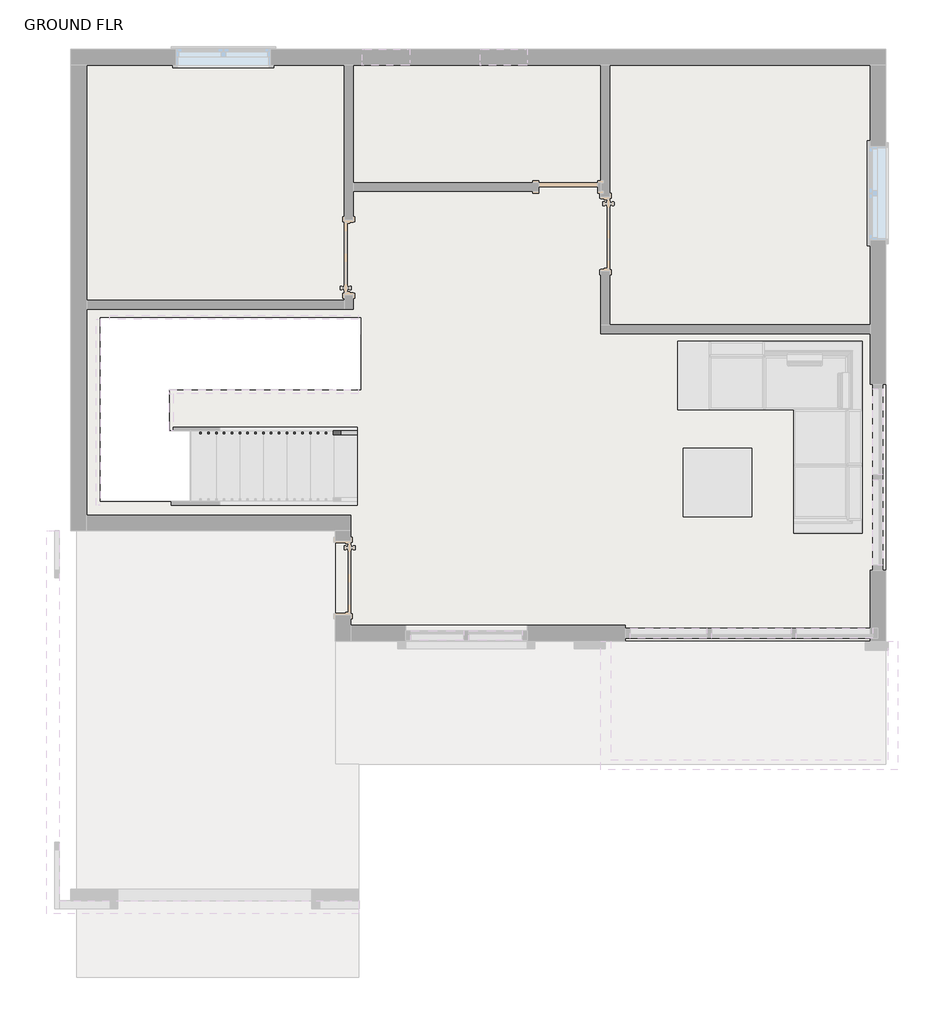
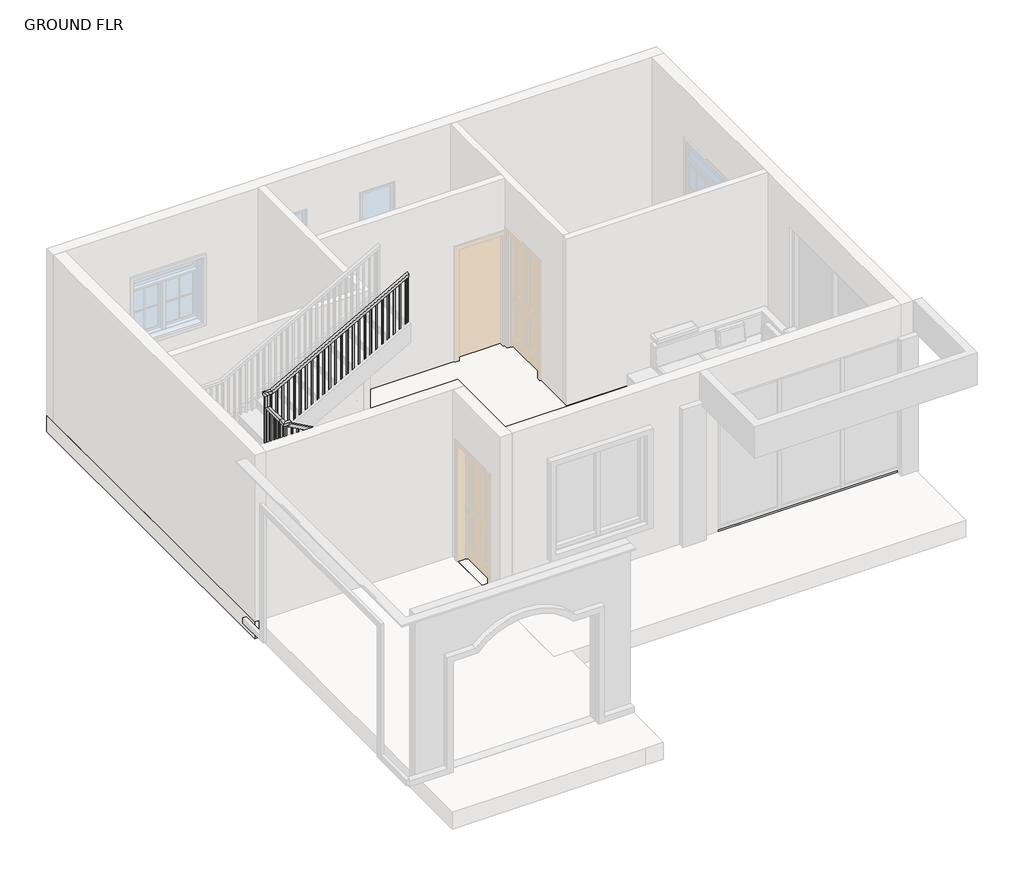
# One storey, part 2 of 3: 3 slabs, 1 beam, 1 railing.
"""IFC4 building model written with IfcOpenShell, lengths in millimetres."""

from ifc_helpers import new_model, si_unit, frame, origin, origin_with_axes, place, context, project, spatial, polyline, outline, extrude, faceted_brep, element, save

model = new_model("IFC4")

# Units and contexts
model_context = context("Model", 3, world=origin())
ifc_project = project(units=[si_unit("LENGTHUNIT", "METRE", prefix="MILLI")], contexts=[model_context])

# Site, building, storey
site = spatial("IfcSite", under=ifc_project)
building = spatial("IfcBuilding", under=site)
storey = spatial("IfcBuildingStorey", under=building, Name="GROUND FLR", Elevation=304.8)

# Beam
placement = place(None, origin())
element("IfcBeam", 1, ObjectType="Concrete-Rectangular Beam : 12 x 24", at=placement, inside=storey, context=model_context, shape_type="Brep", body=[
    faceted_brep([(-11339.0293601, -13183.002305, 304.8), (-11339.0293601, -13487.802305, 304.8), (-8226.1270642, -13487.802305, 304.8), (-8226.1270642, -13183.002305, 304.8), (-11339.0293601, -13183.002305, -304.8), (-11339.0293601, -13183.002305, 0.0), (-8226.1270642, -13183.002305, 0.0), (-8226.1270642, -13183.002305, -304.8), (-11339.0293601, -13487.802305, -304.8), (-8226.1270642, -13487.802305, -304.8), (-11339.0293601, -13487.802305, 0.0), (-8226.1270642, -13487.802305, 0.0)], [[[0, 1, 2, 3]], [[4, 5, 0, 3, 6, 7]], [[8, 4, 7, 9]], [[1, 10, 8, 9, 11, 2]], [[2, 11, 9, 7, 6, 3]], [[1, 0, 5, 4, 8, 10]]]),
])

# Railing
element("IfcRailing", 2, ObjectType="Handrail - Rectangular", at=placement, inside=storey, context=model_context, shape_type="SolidModel", body=[
    faceted_brep([(-7930.9736584, -7598.0396616, 1388.5333333), (-7930.9736584, -7598.0396616, 1330.420221), (-7930.9736584, -7547.2396616, 1330.420221), (-7930.9736584, -7547.2396616, 1388.5333333), (-10293.1736584, -7598.0396616, 2700.8666667), (-10343.9736584, -7598.0396616, 2670.9757765), (-10343.9736584, -7547.2396616, 2670.9757765), (-10293.1736584, -7547.2396616, 2700.8666667), (-10293.1736584, -7598.0396616, 2743.2), (-10343.9736584, -7598.0396616, 2692.4), (-10343.9736584, -7547.2396616, 2692.4), (-10293.1736584, -7547.2396616, 2743.2), (-10420.1736584, -7598.0396616, 2743.2), (-10420.1736584, -7598.0396616, 2692.4), (-10369.3736584, -7547.2396616, 2692.4), (-10369.3736584, -7547.2396616, 2743.2), (-10420.1736584, -7471.0396616, 2743.2), (-10420.1736584, -7471.0396616, 2692.4), (-10369.3736584, -7471.0396616, 2692.4), (-10369.3736584, -7471.0396616, 2743.2), (-10420.1736584, -7090.0396616, 2743.2), (-10420.1736584, -7039.2396616, 2692.4), (-10369.3736584, -7039.2396616, 2692.4), (-10369.3736584, -7090.0396616, 2743.2), (-10420.1736584, -7090.0396616, 2949.5074477), (-10420.1736584, -7039.2396616, 2898.7074477), (-10369.3736584, -7039.2396616, 2898.7074477), (-10369.3736584, -7090.0396616, 2949.5074477), (-10420.1736584, -6963.0396616, 2949.5074477), (-10420.1736584, -6963.0396616, 2898.7074477), (-10369.3736584, -7013.8396616, 2898.7074477), (-10369.3736584, -7013.8396616, 2949.5074477), (-10293.1736584, -6963.0396616, 2949.5074477), (-10280.0100562, -6963.0396616, 2898.7074477), (-10280.0100562, -7013.8396616, 2898.7074477), (-10293.1736584, -7013.8396616, 2949.5074477), (-7921.3270642, -6963.0396616, 4267.2), (-7921.3270642, -7013.8396616, 4267.2), (-7921.3270642, -7013.8396616, 4209.0868876), (-7921.3270642, -6963.0396616, 4209.0868876)], [[[0, 1, 2, 3]], [[1, 0, 4, 5]], [[2, 1, 5, 6]], [[3, 2, 6, 7]], [[0, 3, 7, 4]], [[5, 4, 8, 9]], [[6, 5, 9, 10]], [[7, 6, 10, 11]], [[4, 7, 11, 8]], [[9, 8, 12, 13]], [[10, 9, 13, 14]], [[11, 10, 14, 15]], [[8, 11, 15, 12]], [[13, 12, 16, 17]], [[14, 13, 17, 18]], [[15, 14, 18, 19]], [[12, 15, 19, 16]], [[17, 16, 20, 21]], [[18, 17, 21, 22]], [[19, 18, 22, 23]], [[16, 19, 23, 20]], [[21, 20, 24, 25]], [[22, 21, 25, 26]], [[23, 22, 26, 27]], [[20, 23, 27, 24]], [[25, 24, 28, 29]], [[26, 25, 29, 30]], [[27, 26, 30, 31]], [[24, 27, 31, 28]], [[29, 28, 32, 33]], [[30, 29, 33, 34]], [[31, 30, 34, 35]], [[28, 31, 35, 32]], [[36, 37, 38, 39]], [[33, 32, 36, 39]], [[34, 33, 39, 38]], [[35, 34, 38, 37]], [[32, 35, 37, 36]]]),
    extrude(outline(polyline([(4194.9082242, -7946.8486584), (4184.3248909, -7965.8986584), (3183.4666667, -7965.8986584), (3183.4666667, -7946.8486584), (4194.9082242, -7946.8486584)])), frame((0.0, -6997.9646616, 0.0), z_axis=(0.0, 1.0, 0.0), x_axis=(0.0, 0.0, 1.0)), (0.0, 0.0, 1.0), 19.05),
    extrude(outline(polyline([(4138.4637797, -8048.4486584), (4127.8804464, -8067.4986584), (3183.4666667, -8067.4986584), (3183.4666667, -8048.4486584), (4138.4637797, -8048.4486584)])), frame((0.0, -6997.9646616, 0.0), z_axis=(0.0, 1.0, 0.0), x_axis=(0.0, 0.0, 1.0)), (0.0, 0.0, 1.0), 19.05),
    extrude(outline(polyline([(4082.0193353, -8150.0486584), (4071.436002, -8169.0986584), (3183.4666667, -8169.0986584), (3183.4666667, -8150.0486584), (4082.0193353, -8150.0486584)])), frame((0.0, -6997.9646616, 0.0), z_axis=(0.0, 1.0, 0.0), x_axis=(0.0, 0.0, 1.0)), (0.0, 0.0, 1.0), 19.05),
    extrude(outline(polyline([(4025.5748909, -8251.6486584), (4014.9915575, -8270.6986584), (3014.1333333, -8270.6986584), (3014.1333333, -8251.6486584), (4025.5748909, -8251.6486584)])), frame((0.0, -6997.9646616, 0.0), z_axis=(0.0, 1.0, 0.0), x_axis=(0.0, 0.0, 1.0)), (0.0, 0.0, 1.0), 19.05),
    extrude(outline(polyline([(3969.1304464, -8353.2486584), (3958.5471131, -8372.2986584), (3014.1333333, -8372.2986584), (3014.1333333, -8353.2486584), (3969.1304464, -8353.2486584)])), frame((0.0, -6997.9646616, 0.0), z_axis=(0.0, 1.0, 0.0), x_axis=(0.0, 0.0, 1.0)), (0.0, 0.0, 1.0), 19.05),
    extrude(outline(polyline([(3912.686002, -8454.8486584), (3902.1026686, -8473.8986584), (3014.1333333, -8473.8986584), (3014.1333333, -8454.8486584), (3912.686002, -8454.8486584)])), frame((0.0, -6997.9646616, 0.0), z_axis=(0.0, 1.0, 0.0), x_axis=(0.0, 0.0, 1.0)), (0.0, 0.0, 1.0), 19.05),
    extrude(outline(polyline([(3856.2415575, -8556.4486584), (3845.6582242, -8575.4986584), (2844.8, -8575.4986584), (2844.8, -8556.4486584), (3856.2415575, -8556.4486584)])), frame((0.0, -6997.9646616, 0.0), z_axis=(0.0, 1.0, 0.0), x_axis=(0.0, 0.0, 1.0)), (0.0, 0.0, 1.0), 19.05),
    extrude(outline(polyline([(3799.7971131, -8658.0486584), (3789.2137797, -8677.0986584), (2844.8, -8677.0986584), (2844.8, -8658.0486584), (3799.7971131, -8658.0486584)])), frame((0.0, -6997.9646616, 0.0), z_axis=(0.0, 1.0, 0.0), x_axis=(0.0, 0.0, 1.0)), (0.0, 0.0, 1.0), 19.05),
    extrude(outline(polyline([(3743.3526686, -8759.6486584), (3732.7693353, -8778.6986584), (2844.8, -8778.6986584), (2844.8, -8759.6486584), (3743.3526686, -8759.6486584)])), frame((0.0, -6997.9646616, 0.0), z_axis=(0.0, 1.0, 0.0), x_axis=(0.0, 0.0, 1.0)), (0.0, 0.0, 1.0), 19.05),
    extrude(outline(polyline([(3686.9082242, -8861.2486584), (3676.3248909, -8880.2986584), (2675.4666667, -8880.2986584), (2675.4666667, -8861.2486584), (3686.9082242, -8861.2486584)])), frame((0.0, -6997.9646616, 0.0), z_axis=(0.0, 1.0, 0.0), x_axis=(0.0, 0.0, 1.0)), (0.0, 0.0, 1.0), 19.05),
    extrude(outline(polyline([(3630.4637797, -8962.8486584), (3619.8804464, -8981.8986584), (2675.4666667, -8981.8986584), (2675.4666667, -8962.8486584), (3630.4637797, -8962.8486584)])), frame((0.0, -6997.9646616, 0.0), z_axis=(0.0, 1.0, 0.0), x_axis=(0.0, 0.0, 1.0)), (0.0, 0.0, 1.0), 19.05),
    extrude(outline(polyline([(3574.0193353, -9064.4486584), (3563.436002, -9083.4986584), (2675.4666667, -9083.4986584), (2675.4666667, -9064.4486584), (3574.0193353, -9064.4486584)])), frame((0.0, -6997.9646616, 0.0), z_axis=(0.0, 1.0, 0.0), x_axis=(0.0, 0.0, 1.0)), (0.0, 0.0, 1.0), 19.05),
    extrude(outline(polyline([(3517.5748909, -9166.0486584), (3506.9915575, -9185.0986584), (2506.1333333, -9185.0986584), (2506.1333333, -9166.0486584), (3517.5748909, -9166.0486584)])), frame((0.0, -6997.9646616, 0.0), z_axis=(0.0, 1.0, 0.0), x_axis=(0.0, 0.0, 1.0)), (0.0, 0.0, 1.0), 19.05),
    extrude(outline(polyline([(3461.1304464, -9267.6486584), (3450.5471131, -9286.6986584), (2506.1333333, -9286.6986584), (2506.1333333, -9267.6486584), (3461.1304464, -9267.6486584)])), frame((0.0, -6997.9646616, 0.0), z_axis=(0.0, 1.0, 0.0), x_axis=(0.0, 0.0, 1.0)), (0.0, 0.0, 1.0), 19.05),
    extrude(outline(polyline([(3404.686002, -9369.2486584), (3394.1026686, -9388.2986584), (2506.1333333, -9388.2986584), (2506.1333333, -9369.2486584), (3404.686002, -9369.2486584)])), frame((0.0, -6997.9646616, 0.0), z_axis=(0.0, 1.0, 0.0), x_axis=(0.0, 0.0, 1.0)), (0.0, 0.0, 1.0), 19.05),
    extrude(outline(polyline([(3348.2415575, -9470.8486584), (3337.6582242, -9489.8986584), (2336.8, -9489.8986584), (2336.8, -9470.8486584), (3348.2415575, -9470.8486584)])), frame((0.0, -6997.9646616, 0.0), z_axis=(0.0, 1.0, 0.0), x_axis=(0.0, 0.0, 1.0)), (0.0, 0.0, 1.0), 19.05),
    extrude(outline(polyline([(3291.7971131, -9572.4486584), (3281.2137797, -9591.4986584), (2336.8, -9591.4986584), (2336.8, -9572.4486584), (3291.7971131, -9572.4486584)])), frame((0.0, -6997.9646616, 0.0), z_axis=(0.0, 1.0, 0.0), x_axis=(0.0, 0.0, 1.0)), (0.0, 0.0, 1.0), 19.05),
    extrude(outline(polyline([(3235.3526686, -9674.0486584), (3224.7693353, -9693.0986584), (2336.8, -9693.0986584), (2336.8, -9674.0486584), (3235.3526686, -9674.0486584)])), frame((0.0, -6997.9646616, 0.0), z_axis=(0.0, 1.0, 0.0), x_axis=(0.0, 0.0, 1.0)), (0.0, 0.0, 1.0), 19.05),
    extrude(outline(polyline([(3178.9082242, -9775.6486584), (3168.3248909, -9794.6986584), (2167.4666667, -9794.6986584), (2167.4666667, -9775.6486584), (3178.9082242, -9775.6486584)])), frame((0.0, -6997.9646616, 0.0), z_axis=(0.0, 1.0, 0.0), x_axis=(0.0, 0.0, 1.0)), (0.0, 0.0, 1.0), 19.05),
    extrude(outline(polyline([(3122.4637797, -9877.2486584), (3111.8804464, -9896.2986584), (2167.4666667, -9896.2986584), (2167.4666667, -9877.2486584), (3122.4637797, -9877.2486584)])), frame((0.0, -6997.9646616, 0.0), z_axis=(0.0, 1.0, 0.0), x_axis=(0.0, 0.0, 1.0)), (0.0, 0.0, 1.0), 19.05),
    extrude(outline(polyline([(3066.0193353, -9978.8486584), (3055.436002, -9997.8986584), (2167.4666667, -9997.8986584), (2167.4666667, -9978.8486584), (3066.0193353, -9978.8486584)])), frame((0.0, -6997.9646616, 0.0), z_axis=(0.0, 1.0, 0.0), x_axis=(0.0, 0.0, 1.0)), (0.0, 0.0, 1.0), 19.05),
    extrude(outline(polyline([(3009.5748909, -10080.4486584), (2998.9915575, -10099.4986584), (1998.1333333, -10099.4986584), (1998.1333333, -10080.4486584), (3009.5748909, -10080.4486584)])), frame((0.0, -6997.9646616, 0.0), z_axis=(0.0, 1.0, 0.0), x_axis=(0.0, 0.0, 1.0)), (0.0, 0.0, 1.0), 19.05),
    extrude(outline(polyline([(2953.1304464, -10182.0486584), (2942.5471131, -10201.0986584), (1998.1333333, -10201.0986584), (1998.1333333, -10182.0486584), (2953.1304464, -10182.0486584)])), frame((0.0, -6997.9646616, 0.0), z_axis=(0.0, 1.0, 0.0), x_axis=(0.0, 0.0, 1.0)), (0.0, 0.0, 1.0), 19.05),
    extrude(outline(polyline([(2896.686002, -10283.6486584), (2886.1026686, -10302.6986584), (1998.1333333, -10302.6986584), (1998.1333333, -10283.6486584), (2896.686002, -10283.6486584)])), frame((0.0, -6997.9646616, 0.0), z_axis=(0.0, 1.0, 0.0), x_axis=(0.0, 0.0, 1.0)), (0.0, 0.0, 1.0), 19.05),
    extrude(outline(polyline([(-10385.2486584, -7074.1646616), (-10404.2986584, -7074.1646616), (-10404.2986584, -7055.1146616), (-10385.2486584, -7055.1146616), (-10385.2486584, -7074.1646616)])), frame((0.0, 0.0, 1828.8), z_axis=(0.0, 0.0, 1.0), x_axis=(1.0, 0.0, 0.0)), (0.0, 0.0, 1.0), 1069.9074477),
    extrude(outline(polyline([(-10385.2486584, -7175.7646616), (-10404.2986584, -7175.7646616), (-10404.2986584, -7156.7146616), (-10385.2486584, -7156.7146616), (-10385.2486584, -7175.7646616)])), frame((0.0, 0.0, 1828.8), z_axis=(0.0, 0.0, 1.0), x_axis=(1.0, 0.0, 0.0)), (0.0, 0.0, 1.0), 863.6),
    extrude(outline(polyline([(-10385.2486584, -7277.3646616), (-10404.2986584, -7277.3646616), (-10404.2986584, -7258.3146616), (-10385.2486584, -7258.3146616), (-10385.2486584, -7277.3646616)])), frame((0.0, 0.0, 1828.8), z_axis=(0.0, 0.0, 1.0), x_axis=(1.0, 0.0, 0.0)), (0.0, 0.0, 1.0), 863.6),
    extrude(outline(polyline([(-10385.2486584, -7378.9646616), (-10404.2986584, -7378.9646616), (-10404.2986584, -7359.9146616), (-10385.2486584, -7359.9146616), (-10385.2486584, -7378.9646616)])), frame((0.0, 0.0, 1828.8), z_axis=(0.0, 0.0, 1.0), x_axis=(1.0, 0.0, 0.0)), (0.0, 0.0, 1.0), 863.6),
    extrude(outline(polyline([(-10385.2486584, -7480.5646616), (-10404.2986584, -7480.5646616), (-10404.2986584, -7461.5146616), (-10385.2486584, -7461.5146616), (-10385.2486584, -7480.5646616)])), frame((0.0, 0.0, 1828.8), z_axis=(0.0, 0.0, 1.0), x_axis=(1.0, 0.0, 0.0)), (0.0, 0.0, 1.0), 863.6),
    extrude(outline(polyline([(-10359.8486584, -7563.1146616), (-10359.8486584, -7582.1646616), (-10378.8986584, -7582.1646616), (-10378.8986584, -7563.1146616), (-10359.8486584, -7563.1146616)])), frame((0.0, 0.0, 1828.8), z_axis=(0.0, 0.0, 1.0), x_axis=(1.0, 0.0, 0.0)), (0.0, 0.0, 1.0), 863.6),
    extrude(outline(polyline([(2623.3507765, -10258.2486584), (2633.9341099, -10277.2986584), (1659.4666667, -10277.2986584), (1659.4666667, -10258.2486584), (2623.3507765, -10258.2486584)])), frame((0.0, -7582.1646616, 0.0), z_axis=(0.0, 1.0, 0.0), x_axis=(0.0, 0.0, 1.0)), (0.0, 0.0, 1.0), 19.05),
    extrude(outline(polyline([(2566.9063321, -10156.6486584), (2577.4896654, -10175.6986584), (1659.4666667, -10175.6986584), (1659.4666667, -10156.6486584), (2566.9063321, -10156.6486584)])), frame((0.0, -7582.1646616, 0.0), z_axis=(0.0, 1.0, 0.0), x_axis=(0.0, 0.0, 1.0)), (0.0, 0.0, 1.0), 19.05),
    extrude(outline(polyline([(2510.4618876, -10055.0486584), (2521.045221, -10074.0986584), (1659.4666667, -10074.0986584), (1659.4666667, -10055.0486584), (2510.4618876, -10055.0486584)])), frame((0.0, -7582.1646616, 0.0), z_axis=(0.0, 1.0, 0.0), x_axis=(0.0, 0.0, 1.0)), (0.0, 0.0, 1.0), 19.05),
    extrude(outline(polyline([(2454.0174432, -9953.4486584), (2464.6007765, -9972.4986584), (1490.1333333, -9972.4986584), (1490.1333333, -9953.4486584), (2454.0174432, -9953.4486584)])), frame((0.0, -7582.1646616, 0.0), z_axis=(0.0, 1.0, 0.0), x_axis=(0.0, 0.0, 1.0)), (0.0, 0.0, 1.0), 19.05),
    extrude(outline(polyline([(2397.5729988, -9851.8486584), (2408.1563321, -9870.8986584), (1490.1333333, -9870.8986584), (1490.1333333, -9851.8486584), (2397.5729988, -9851.8486584)])), frame((0.0, -7582.1646616, 0.0), z_axis=(0.0, 1.0, 0.0), x_axis=(0.0, 0.0, 1.0)), (0.0, 0.0, 1.0), 19.05),
    extrude(outline(polyline([(2341.1285543, -9750.2486584), (2351.7118876, -9769.2986584), (1490.1333333, -9769.2986584), (1490.1333333, -9750.2486584), (2341.1285543, -9750.2486584)])), frame((0.0, -7582.1646616, 0.0), z_axis=(0.0, 1.0, 0.0), x_axis=(0.0, 0.0, 1.0)), (0.0, 0.0, 1.0), 19.05),
    extrude(outline(polyline([(2284.6841099, -9648.6486584), (2295.2674432, -9667.6986584), (1320.8, -9667.6986584), (1320.8, -9648.6486584), (2284.6841099, -9648.6486584)])), frame((0.0, -7582.1646616, 0.0), z_axis=(0.0, 1.0, 0.0), x_axis=(0.0, 0.0, 1.0)), (0.0, 0.0, 1.0), 19.05),
    extrude(outline(polyline([(2228.2396654, -9547.0486584), (2238.8229988, -9566.0986584), (1320.8, -9566.0986584), (1320.8, -9547.0486584), (2228.2396654, -9547.0486584)])), frame((0.0, -7582.1646616, 0.0), z_axis=(0.0, 1.0, 0.0), x_axis=(0.0, 0.0, 1.0)), (0.0, 0.0, 1.0), 19.05),
    extrude(outline(polyline([(2171.795221, -9445.4486584), (2182.3785543, -9464.4986584), (1320.8, -9464.4986584), (1320.8, -9445.4486584), (2171.795221, -9445.4486584)])), frame((0.0, -7582.1646616, 0.0), z_axis=(0.0, 1.0, 0.0), x_axis=(0.0, 0.0, 1.0)), (0.0, 0.0, 1.0), 19.05),
    extrude(outline(polyline([(2115.3507765, -9343.8486584), (2125.9341099, -9362.8986584), (1151.4666667, -9362.8986584), (1151.4666667, -9343.8486584), (2115.3507765, -9343.8486584)])), frame((0.0, -7582.1646616, 0.0), z_axis=(0.0, 1.0, 0.0), x_axis=(0.0, 0.0, 1.0)), (0.0, 0.0, 1.0), 19.05),
    extrude(outline(polyline([(2058.9063321, -9242.2486584), (2069.4896654, -9261.2986584), (1151.4666667, -9261.2986584), (1151.4666667, -9242.2486584), (2058.9063321, -9242.2486584)])), frame((0.0, -7582.1646616, 0.0), z_axis=(0.0, 1.0, 0.0), x_axis=(0.0, 0.0, 1.0)), (0.0, 0.0, 1.0), 19.05),
    extrude(outline(polyline([(2002.4618876, -9140.6486584), (2013.045221, -9159.6986584), (1151.4666667, -9159.6986584), (1151.4666667, -9140.6486584), (2002.4618876, -9140.6486584)])), frame((0.0, -7582.1646616, 0.0), z_axis=(0.0, 1.0, 0.0), x_axis=(0.0, 0.0, 1.0)), (0.0, 0.0, 1.0), 19.05),
    extrude(outline(polyline([(1946.0174432, -9039.0486584), (1956.6007765, -9058.0986584), (982.1333333, -9058.0986584), (982.1333333, -9039.0486584), (1946.0174432, -9039.0486584)])), frame((0.0, -7582.1646616, 0.0), z_axis=(0.0, 1.0, 0.0), x_axis=(0.0, 0.0, 1.0)), (0.0, 0.0, 1.0), 19.05),
    extrude(outline(polyline([(1889.5729988, -8937.4486584), (1900.1563321, -8956.4986584), (982.1333333, -8956.4986584), (982.1333333, -8937.4486584), (1889.5729988, -8937.4486584)])), frame((0.0, -7582.1646616, 0.0), z_axis=(0.0, 1.0, 0.0), x_axis=(0.0, 0.0, 1.0)), (0.0, 0.0, 1.0), 19.05),
    extrude(outline(polyline([(1833.1285543, -8835.8486584), (1843.7118876, -8854.8986584), (982.1333333, -8854.8986584), (982.1333333, -8835.8486584), (1833.1285543, -8835.8486584)])), frame((0.0, -7582.1646616, 0.0), z_axis=(0.0, 1.0, 0.0), x_axis=(0.0, 0.0, 1.0)), (0.0, 0.0, 1.0), 19.05),
    extrude(outline(polyline([(1776.6841099, -8734.2486584), (1787.2674432, -8753.2986584), (812.8, -8753.2986584), (812.8, -8734.2486584), (1776.6841099, -8734.2486584)])), frame((0.0, -7582.1646616, 0.0), z_axis=(0.0, 1.0, 0.0), x_axis=(0.0, 0.0, 1.0)), (0.0, 0.0, 1.0), 19.05),
    extrude(outline(polyline([(1720.2396654, -8632.6486584), (1730.8229988, -8651.6986584), (812.8, -8651.6986584), (812.8, -8632.6486584), (1720.2396654, -8632.6486584)])), frame((0.0, -7582.1646616, 0.0), z_axis=(0.0, 1.0, 0.0), x_axis=(0.0, 0.0, 1.0)), (0.0, 0.0, 1.0), 19.05),
    extrude(outline(polyline([(1663.795221, -8531.0486584), (1674.3785543, -8550.0986584), (812.8, -8550.0986584), (812.8, -8531.0486584), (1663.795221, -8531.0486584)])), frame((0.0, -7582.1646616, 0.0), z_axis=(0.0, 1.0, 0.0), x_axis=(0.0, 0.0, 1.0)), (0.0, 0.0, 1.0), 19.05),
    extrude(outline(polyline([(1607.3507765, -8429.4486584), (1617.9341099, -8448.4986584), (643.4666667, -8448.4986584), (643.4666667, -8429.4486584), (1607.3507765, -8429.4486584)])), frame((0.0, -7582.1646616, 0.0), z_axis=(0.0, 1.0, 0.0), x_axis=(0.0, 0.0, 1.0)), (0.0, 0.0, 1.0), 19.05),
    extrude(outline(polyline([(1550.9063321, -8327.8486584), (1561.4896654, -8346.8986584), (643.4666667, -8346.8986584), (643.4666667, -8327.8486584), (1550.9063321, -8327.8486584)])), frame((0.0, -7582.1646616, 0.0), z_axis=(0.0, 1.0, 0.0), x_axis=(0.0, 0.0, 1.0)), (0.0, 0.0, 1.0), 19.05),
    extrude(outline(polyline([(1494.4618876, -8226.2486584), (1505.045221, -8245.2986584), (643.4666667, -8245.2986584), (643.4666667, -8226.2486584), (1494.4618876, -8226.2486584)])), frame((0.0, -7582.1646616, 0.0), z_axis=(0.0, 1.0, 0.0), x_axis=(0.0, 0.0, 1.0)), (0.0, 0.0, 1.0), 19.05),
    extrude(outline(polyline([(1438.0174432, -8124.6486584), (1448.6007765, -8143.6986584), (474.1333333, -8143.6986584), (474.1333333, -8124.6486584), (1438.0174432, -8124.6486584)])), frame((0.0, -7582.1646616, 0.0), z_axis=(0.0, 1.0, 0.0), x_axis=(0.0, 0.0, 1.0)), (0.0, 0.0, 1.0), 19.05),
    extrude(outline(polyline([(1381.5729988, -8023.0486584), (1392.1563321, -8042.0986584), (474.1333333, -8042.0986584), (474.1333333, -8023.0486584), (1381.5729988, -8023.0486584)])), frame((0.0, -7582.1646616, 0.0), z_axis=(0.0, 1.0, 0.0), x_axis=(0.0, 0.0, 1.0)), (0.0, 0.0, 1.0), 19.05),
    extrude(outline(polyline([(-10385.2486584, -6997.9646616), (-10404.2986584, -6997.9646616), (-10404.2986584, -6978.9146616), (-10385.2486584, -6978.9146616), (-10385.2486584, -6997.9646616)])), frame((0.0, 0.0, 1828.8), z_axis=(0.0, 0.0, 1.0), x_axis=(1.0, 0.0, 0.0)), (0.0, 0.0, 1.0), 1069.9074477),
    extrude(outline(polyline([(-10385.2486584, -7563.1146616), (-10385.2486584, -7582.1646616), (-10404.2986584, -7582.1646616), (-10404.2986584, -7563.1146616), (-10385.2486584, -7563.1146616)])), frame((0.0, 0.0, 1828.8), z_axis=(0.0, 0.0, 1.0), x_axis=(1.0, 0.0, 0.0)), (0.0, 0.0, 1.0), 863.6),
    extrude(outline(polyline([(4209.0868876, -7921.3270642), (4198.5035543, -7940.3770642), (3183.4666667, -7940.3770642), (3183.4666667, -7921.3270642), (4209.0868876, -7921.3270642)])), frame((0.0, -6997.9646616, 0.0), z_axis=(0.0, 1.0, 0.0), x_axis=(0.0, 0.0, 1.0)), (0.0, 0.0, 1.0), 19.05),
    extrude(outline(polyline([(1330.420221, -7930.9736584), (1341.0035543, -7950.0236584), (474.1333333, -7950.0236584), (474.1333333, -7930.9736584), (1330.420221, -7930.9736584)])), frame((0.0, -7582.1646616, 0.0), z_axis=(0.0, 1.0, 0.0), x_axis=(0.0, 0.0, 1.0)), (0.0, 0.0, 1.0), 19.05),
])

# Slabs
element("IfcSlab", 3, ObjectType="FLOORING 1'", at=placement, inside=storey, context=model_context, shape_type="SweptSolid", body=[
    extrude(outline(polyline([(-1079.3236584, -10271.3896616), (-8216.7236584, -10271.3896616), (-8216.7236584, -8842.6396616), (-11645.7236584, -8842.6396616), (-11645.7236584, -2600.5896616), (-1079.3236584, -2600.5896616), (-1079.3236584, -10271.3896616)]), holes=[polyline([(-11264.7236584, -6080.3896616), (-11264.7236584, -8461.6396616), (-7930.9736584, -8461.6396616), (-7930.9736584, -7547.2396616), (-10369.3736584, -7547.2396616), (-10369.3736584, -7013.8396616), (-7889.5770642, -7013.8396616), (-7889.5770642, -6080.3896616), (-11264.7236584, -6080.3896616)])]), origin_with_axes(), (0.0, 0.0, 1.0), 304.8),
])
element("IfcSlab", 4, ObjectType="Generic - 12\"", at=placement, inside=storey, context=model_context, shape_type="SweptSolid", body=[
    extrude(outline(polyline([(-4797.1270642, -2868.8747117), (-4797.1270642, -5993.0747117), (-7946.7270642, -5993.0747117), (-7946.7270642, -2868.8747117), (-4797.1270642, -2868.8747117)])), frame((0.0, 0.0, -304.8), z_axis=(0.0, 0.0, 1.0), x_axis=(1.0, 0.0, 0.0)), (0.0, 0.0, 1.0), 304.8),
])
element("IfcSlab", 5, ObjectType="Generic - 12\"", at=placement, inside=storey, context=model_context, shape_type="SweptSolid", body=[
    extrude(outline(polyline([(-1351.9658472, -2868.8747117), (-1351.9658472, -5993.0747117), (-4492.3270642, -5993.0747117), (-4492.3270642, -2868.8747117), (-1351.9658472, -2868.8747117)])), frame((0.0, 0.0, -304.8), z_axis=(0.0, 0.0, 1.0), x_axis=(1.0, 0.0, 0.0)), (0.0, 0.0, 1.0), 304.8),
])

save(model, "model.ifc")

# Revit data of these elements
# Type "Concrete-Rectangular Beam : 12 x 24"
#   Assembly Code = "B10"
#   Length [instance default] = 5' - 0"
#   b = 1' - 0"
#   h = 2' - 0"
#   Structural Material [instance default] = Concrete, Cast-in-Place gray
# Type "Handrail - Rectangular"
#   Assembly Code = "C2010400"
#   built-in parameter 1008612 = 0.0416667 (stored number, unit not read)
#   built-in parameter 1008611 = 0.0416667 (stored number, unit not read)
#   built-in parameter 1008609 = 0.333333 (stored number, unit not read)
#   built-in parameter 1008604 = 0.166667 (stored number, unit not read)
#   built-in parameter 1008603 = 0.166667 (stored number, unit not read)
#   Railing Height = 3' - 0"
#   built-in parameter 1008630 = 2
#   built-in parameter 1008610 = 2
#   built-in parameter 1008618 = Baluster - Square : 3/4"
# Type "FLOORING 1'"
#   Assembly Code = "B1010"
#   Function = 0
#   Layers, outside or top first: 1' - 0" "MARBLE FLOORING 6\"" (function 1)
# Type "Generic - 12\""
#   Assembly Code = "B1010"
#   Function = 0
#   Layers, outside or top first: 1' - 0" no material (function 1)
# Element 1 (IfcBeam, "Concrete-Rectangular Beam : 12 x 24")
#   Structural Material = Concrete, Cast-in-Place gray
#   Phase Created = New Construction
#   Materials on its faces: "Concrete, Cast-in-Place gray"
# Element 2 (IfcRailing, "Handrail - Rectangular")
#   Phase Created = New Construction
# Element 3 (IfcSlab, "FLOORING 1'")
#   built-in parameter 1001955 = -1.5708 (stored number, unit not read)
#   Height Offset From Level = 0' - 0"
#   Phase Created = New Construction
#   Materials on its faces: "MARBLE FLOORING 6\""
# Elements 4, 5 (IfcSlab, "Generic - 12\"")
#   Height Offset From Level = -1' - 0"
#   built-in parameter 1001954 = 1
#   Phase Created = New Construction
#   Materials on its faces: "Default Floor"
# Materials
#   "Concrete, Cast-in-Place gray": class "Concrete", colour RGB 192 192 192, transparency 0, Description = "Cast-in-place concrete", Cost = 0
#   "MARBLE FLOORING 6\"": class "Generic", colour RGB 120 120 120, transparency 0, Cost = 0
#   "Default Floor": colour RGB 128 128 128, transparency 0, Cost = 0
